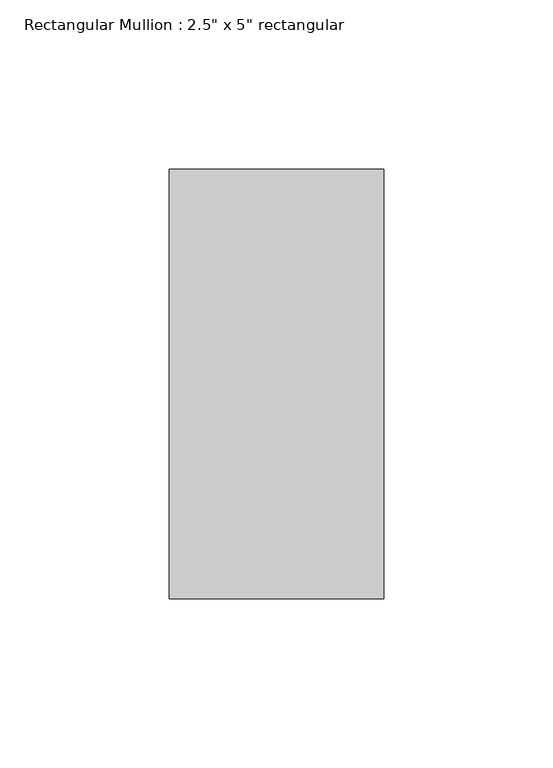
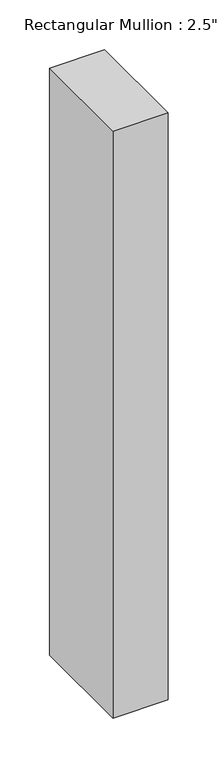
"""IFC4 building model written with IfcOpenShell, lengths in millimetres: member geometry."""

from ifc_helpers import new_model, si_unit, frame, origin, place, context, project, spatial, polyline, outline, extrude, source, transform, mapped, element, save


def member_20537117(model_context):
    return source(origin(), model_context, "Body", "SweptSolid", [
        extrude(outline(polyline([(0.0, 63.5), (0.0, -63.5), (-63.5, -63.5), (-63.5, 63.5), (0.0, 63.5)])), frame((0.0, 0.0, -717.5668761), z_axis=(0.0, 0.0, 1.0), x_axis=(1.0, 0.0, 0.0)), (0.0, 0.0, 1.0), 717.5668761),
    ])


if __name__ == "__main__":
    model = new_model("IFC4")
    model_context = context("Model", 3, world=origin())
    ifc_project = project(units=[si_unit("LENGTHUNIT", "METRE", prefix="MILLI")], contexts=[model_context])
    site = spatial("IfcSite", under=ifc_project)
    building = spatial("IfcBuilding", under=site)
    placement = place(None, origin())
    member_shape = member_20537117(model_context)
    element("IfcMember", 1, ObjectType="Rectangular Mullion : 2.5\" x 5\" rectangular", at=placement, inside=building, context=model_context, shape_type="MappedRepresentation", body=[
        mapped(member_shape, transform((0.0, 0.0, 0.0), x_axis=(1.0, 0.0, 0.0), y_axis=(0.0, 1.0, 0.0), z_axis=(0.0, 0.0, 1.0))),
    ])
    save(model, "model.ifc")

# Revit data of these elements
# Type "Rectangular Mullion : 2.5\" x 5\" rectangular"
#   built-in parameter 1007304 = 0.416667 (stored number, unit not read)
#   built-in parameter 1007301 = 0.104167 (stored number, unit not read)
#   built-in parameter 1007300 = 0.104167 (stored number, unit not read)
# Element 1 (IfcMember, "Rectangular Mullion : 2.5\" x 5\" rectangular")
#   Materials on its faces: "Aluminum"
# Materials
#   "Aluminum": class "Metal", colour RGB 247 247 247, transparency 0, Description = "Aluminum 6061", Cost = 0
